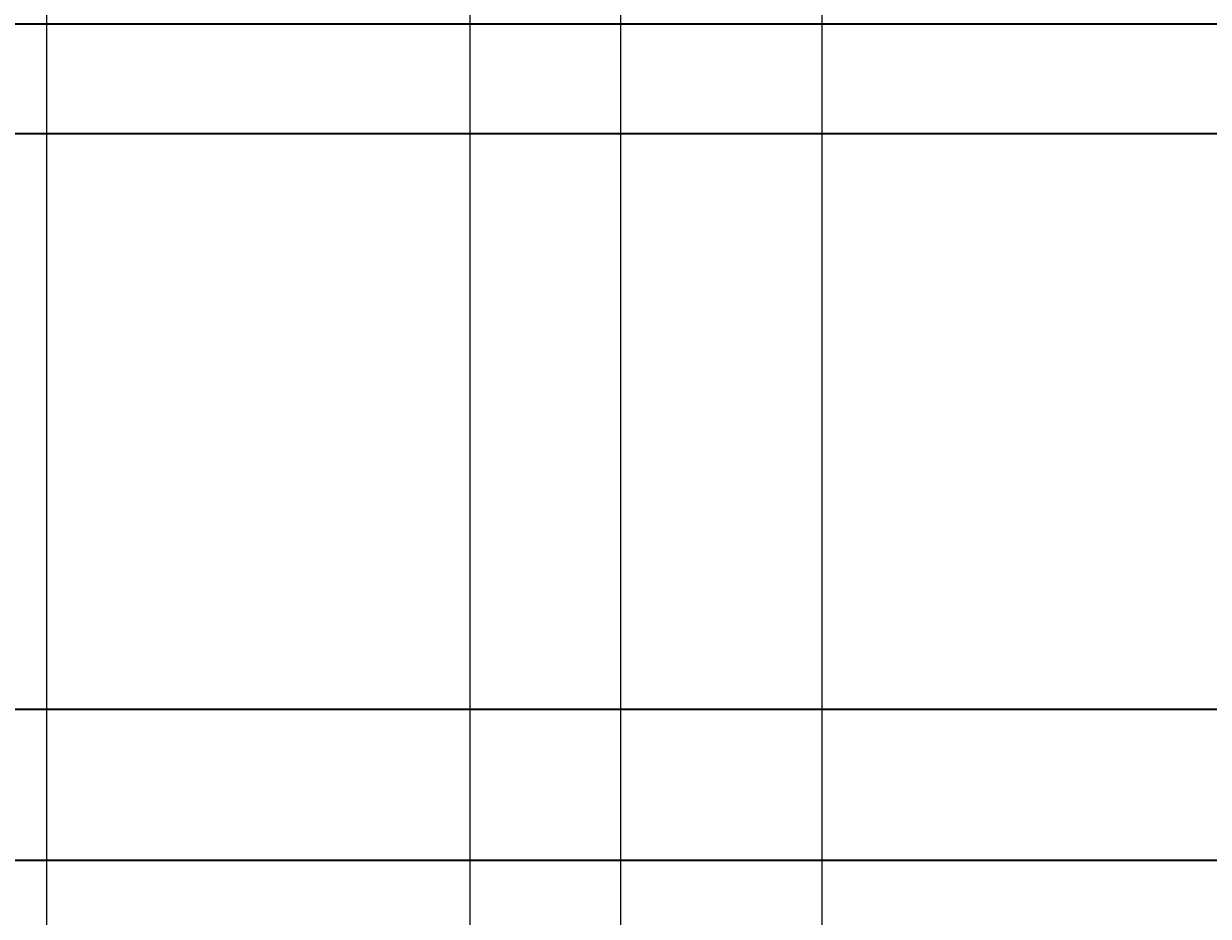
# Model space of a CAD drawing. Units: inches. Extents: x -6 to 289, y -8 to 323.
# Tile 86 of 107: x 126 to 150, y 276 to 294. Entities that reach past the tile are written whole.
import ezdxf

# ---------------------------------------------------------------- set-up
doc = ezdxf.new("R2010")
doc.units = ezdxf.units.IN
doc.header["$MEASUREMENT"] = 0
doc.layers.add('A-ANNO-DIMS', color=2, linetype='Continuous', lineweight=18)
doc.layers.add('A-ELEV', color=7, linetype='Continuous', lineweight=35)
doc.styles.get("Standard").update_dxf_attribs({"font": 'arial.ttf'})
doc.dimstyles.get("Standard").update_dxf_attribs({"dimtxt": 0.18, "dimasz": 0.18, "dimexe": 0.18, "dimexo": 0.0625, "dimgap": 0.09, "dimtad": 0, "dimtih": 1, "dimtoh": 1, "dimdec": 4, "dimzin": 0, "dimdsep": 46, "dimtxsty": 'Standard', "dimcen": 0.09, "dimadec": 0, "dimazin": 0, "dimtfac": 1, "dimtdec": 4, "dimtofl": 0, "dimtmove": 0, "dimatfit": 3, "dimfxl": 1, "dimtolj": 1, "dimtzin": 0, "dimarcsym": 0})

# ---------------------------------------------------------------- blocks, each defined once
blk = doc.blocks.new('*D10')
at = {"layer": 'A-ANNO-DIMS', "color": 0, "lineweight": -2, "transparency": 16777216}
for p, q in [((115.164, 307.351), (115.164, 322.969)), ((126.883, 226.717), (126.883, 322.969)), ((115.344, 322.789), (120.639, 322.789)), ((126.703, 322.789), (121.408, 322.789))]:
    blk.add_line(p, q, dxfattribs=at)
at = {"layer": 'A-ANNO-DIMS', "color": 0, "transparency": 16777216}
for points in [[(115.344, 322.819), (115.344, 322.759), (115.164, 322.789)], [(126.703, 322.819), (126.703, 322.759), (126.883, 322.789)]]:
    blk.add_solid(points, dxfattribs=at)
at = {"layer": 'Defpoints', "color": 0, "transparency": 16777216}
for p in [(126.883, 322.789), (115.164, 307.289), (126.883, 226.654)]:
    blk.add_point(p, dxfattribs=at)
at = {"layer": 'A-ANNO-DIMS', "color": 0, "transparency": 16777216, "insert": (121.024, 322.789), "char_height": 0.18, "attachment_point": 5}
blk.add_mtext('\\A1;11.72', dxfattribs=at)
blk = doc.blocks.new('*D11')
at = {"layer": 'A-ANNO-DIMS', "color": 0, "lineweight": -2, "transparency": 16777216}
for p, q in [((126.883, 226.717), (126.883, 322.969)), ((168.883, 226.717), (168.883, 322.969)), ((127.063, 322.789), (147.662, 322.789)), ((168.703, 322.789), (148.105, 322.789))]:
    blk.add_line(p, q, dxfattribs=at)
at = {"layer": 'A-ANNO-DIMS', "color": 0, "transparency": 16777216}
for points in [[(127.063, 322.819), (127.063, 322.759), (126.883, 322.789)], [(168.703, 322.819), (168.703, 322.759), (168.883, 322.789)]]:
    blk.add_solid(points, dxfattribs=at)
at = {"layer": 'Defpoints', "color": 0, "transparency": 16777216}
for p in [(168.883, 322.789), (126.883, 226.654), (168.883, 226.654)]:
    blk.add_point(p, dxfattribs=at)
at = {"layer": 'A-ANNO-DIMS', "color": 0, "transparency": 16777216, "insert": (147.883, 322.789), "char_height": 0.18, "attachment_point": 5}
blk.add_mtext('\\A1;42', dxfattribs=at)
blk = doc.blocks.new('*D27')
at = {"layer": 'A-ANNO-DIMS', "color": 0, "lineweight": -2, "transparency": 16777216}
for p, q in [((19.226, 307.289), (288.653, 307.289)), ((288.473, 307.109), (288.473, 277.471)), ((288.473, 247.469), (288.473, 277.107)), ((247.226, 247.289), (288.653, 247.289))]:
    blk.add_line(p, q, dxfattribs=at)
at = {"layer": 'A-ANNO-DIMS', "color": 0, "transparency": 16777216}
for points in [[(288.443, 307.109), (288.503, 307.109), (288.473, 307.289)], [(288.443, 247.469), (288.503, 247.469), (288.473, 247.289)]]:
    blk.add_solid(points, dxfattribs=at)
at = {"layer": 'Defpoints', "color": 0, "transparency": 16777216}
for p in [(19.164, 307.289), (288.473, 307.289), (247.164, 247.289)]:
    blk.add_point(p, dxfattribs=at)
at = {"layer": 'A-ANNO-DIMS', "color": 0, "transparency": 16777216, "insert": (288.473, 277.289), "char_height": 0.18, "attachment_point": 5}
blk.add_mtext('\\A1;60', dxfattribs=at)
blk = doc.blocks.new('*D73')
at = {"layer": 'A-ANNO-DIMS', "color": 0, "lineweight": -2, "transparency": 16777216}
for p, q in [((121.008, 51.148), (121.008, 322.969)), ((135.296, 51.148), (135.296, 322.969)), ((121.188, 322.789), (127.697, 322.789)), ((135.116, 322.789), (128.607, 322.789))]:
    blk.add_line(p, q, dxfattribs=at)
at = {"layer": 'A-ANNO-DIMS', "color": 0, "transparency": 16777216}
for points in [[(121.188, 322.819), (121.188, 322.759), (121.008, 322.789)], [(135.116, 322.819), (135.116, 322.759), (135.296, 322.789)]]:
    blk.add_solid(points, dxfattribs=at)
at = {"layer": 'Defpoints', "color": 0, "transparency": 16777216}
for p in [(135.296, 322.789), (121.008, 51.085), (135.296, 51.085)]:
    blk.add_point(p, dxfattribs=at)
at = {"layer": 'A-ANNO-DIMS', "color": 0, "transparency": 16777216, "insert": (128.152, 322.789), "char_height": 0.18, "attachment_point": 5}
blk.add_mtext('\\A1;14.288', dxfattribs=at)
blk = doc.blocks.new('*D74')
at = {"layer": 'A-ANNO-DIMS', "color": 0, "lineweight": -2, "transparency": 16777216}
for p, q in [((135.296, 51.148), (135.296, 322.969)), ((138.296, 51.148), (138.296, 322.969)), ((135.476, 322.789), (136.647, 322.789)), ((138.116, 322.789), (136.945, 322.789))]:
    blk.add_line(p, q, dxfattribs=at)
at = {"layer": 'A-ANNO-DIMS', "color": 0, "transparency": 16777216}
for points in [[(135.476, 322.819), (135.476, 322.759), (135.296, 322.789)], [(138.116, 322.819), (138.116, 322.759), (138.296, 322.789)]]:
    blk.add_solid(points, dxfattribs=at)
at = {"layer": 'Defpoints', "color": 0, "transparency": 16777216}
for p in [(138.296, 322.789), (135.296, 51.085), (138.296, 51.085)]:
    blk.add_point(p, dxfattribs=at)
at = {"layer": 'A-ANNO-DIMS', "color": 0, "transparency": 16777216, "insert": (136.796, 322.789), "char_height": 0.18, "attachment_point": 5}
blk.add_mtext('\\A1;3', dxfattribs=at)
blk = doc.blocks.new('*D75')
at = {"layer": 'A-ANNO-DIMS', "color": 0, "lineweight": -2, "transparency": 16777216}
for p, q in [((138.296, 51.148), (138.296, 322.969)), ((142.296, 51.148), (142.296, 322.969)), ((138.476, 322.789), (140.144, 322.789)), ((142.116, 322.789), (140.448, 322.789))]:
    blk.add_line(p, q, dxfattribs=at)
at = {"layer": 'A-ANNO-DIMS', "color": 0, "transparency": 16777216}
for points in [[(138.476, 322.819), (138.476, 322.759), (138.296, 322.789)], [(142.116, 322.819), (142.116, 322.759), (142.296, 322.789)]]:
    blk.add_solid(points, dxfattribs=at)
at = {"layer": 'Defpoints', "color": 0, "transparency": 16777216}
for p in [(142.296, 322.789), (138.296, 51.085), (142.296, 51.085)]:
    blk.add_point(p, dxfattribs=at)
at = {"layer": 'A-ANNO-DIMS', "color": 0, "transparency": 16777216, "insert": (140.296, 322.789), "char_height": 0.18, "attachment_point": 5}
blk.add_mtext('\\A1;4', dxfattribs=at)
blk = doc.blocks.new('*D76')
at = {"layer": 'A-ANNO-DIMS', "color": 0, "lineweight": -2, "transparency": 16777216}
for p, q in [((142.296, 51.148), (142.296, 322.969)), ((164.296, 51.148), (164.296, 322.969)), ((142.476, 322.789), (153.076, 322.789)), ((164.116, 322.789), (153.516, 322.789))]:
    blk.add_line(p, q, dxfattribs=at)
at = {"layer": 'A-ANNO-DIMS', "color": 0, "transparency": 16777216}
for points in [[(142.476, 322.819), (142.476, 322.759), (142.296, 322.789)], [(164.116, 322.819), (164.116, 322.759), (164.296, 322.789)]]:
    blk.add_solid(points, dxfattribs=at)
at = {"layer": 'Defpoints', "color": 0, "transparency": 16777216}
for p in [(164.296, 322.789), (142.296, 51.085), (164.296, 51.085)]:
    blk.add_point(p, dxfattribs=at)
at = {"layer": 'A-ANNO-DIMS', "color": 0, "transparency": 16777216, "insert": (153.296, 322.789), "char_height": 0.18, "attachment_point": 5}
blk.add_mtext('\\A1;22', dxfattribs=at)
blk = doc.blocks.new('*D94')
at = {"layer": 'A-ANNO-DIMS', "color": 0, "lineweight": -2, "transparency": 16777216}
for p, q in [((118.164, 159.411), (118.164, 322.969)), ((161.552, 159.411), (161.552, 322.969)), ((118.344, 322.789), (139.46, 322.789)), ((161.372, 322.789), (140.256, 322.789))]:
    blk.add_line(p, q, dxfattribs=at)
at = {"layer": 'A-ANNO-DIMS', "color": 0, "transparency": 16777216}
for points in [[(118.344, 322.819), (118.344, 322.759), (118.164, 322.789)], [(161.372, 322.819), (161.372, 322.759), (161.552, 322.789)]]:
    blk.add_solid(points, dxfattribs=at)
at = {"layer": 'Defpoints', "color": 0, "transparency": 16777216}
for p in [(161.552, 322.789), (118.164, 159.348), (161.552, 159.348)]:
    blk.add_point(p, dxfattribs=at)
at = {"layer": 'A-ANNO-DIMS', "color": 0, "transparency": 16777216, "insert": (139.858, 322.789), "char_height": 0.18, "attachment_point": 5}
blk.add_mtext('\\A1;43.39', dxfattribs=at)
blk = doc.blocks.new('*D107')
at = {"layer": 'A-ANNO-DIMS', "color": 0, "lineweight": -2, "transparency": 16777216}
for p, q in [((118.164, 293.728), (118.164, 322.969)), ((186.984, 291.541), (186.984, 322.969)), ((118.344, 322.789), (152.18, 322.789)), ((186.804, 322.789), (152.967, 322.789))]:
    blk.add_line(p, q, dxfattribs=at)
at = {"layer": 'A-ANNO-DIMS', "color": 0, "transparency": 16777216}
for points in [[(118.344, 322.819), (118.344, 322.759), (118.164, 322.789)], [(186.804, 322.819), (186.804, 322.759), (186.984, 322.789)]]:
    blk.add_solid(points, dxfattribs=at)
at = {"layer": 'Defpoints', "color": 0, "transparency": 16777216}
for p in [(186.984, 322.789), (118.164, 293.666), (186.984, 291.478)]:
    blk.add_point(p, dxfattribs=at)
at = {"layer": 'A-ANNO-DIMS', "color": 0, "transparency": 16777216, "insert": (152.574, 322.789), "char_height": 0.18, "attachment_point": 5}
blk.add_mtext('\\A1;68.82', dxfattribs=at)

msp = doc.modelspace()

# ---------------------------------------------------------------- linework, layer by layer
at = {"layer": 'A-ELEV'}
for points in [[(115.1638, 307.2888), (115.1638, 277.0427), (259.1638, 277.0427), (259.1638, 259.2888)], [(118.1638, 307.2888), (118.1638, 280.0427), (262.1638, 280.0427), (262.1638, 259.2888)], [(255.8036, 291.4781), (118.1638, 291.4781), (118.1638, 293.6657), (255.8036, 293.6657)]]:
    msp.add_lwpolyline(points, dxfattribs=at)

# ---------------------------------------------------------------- dimensions: what is measured, and where the dimension line sits
at = {"layer": 'A-ANNO-DIMS'}
for base, p1, p2, override, picture, middle in [((126.8835, 322.7888), (115.1638, 307.2888), (126.8835, 226.654), {"dimdec": 2, "dimlfac": 1, "dimrnd": 0, "dimzin": 0, "dimdsep": 46, "dimlunit": 2}, '*D10', (121.0236, 322.7888)), ((161.5522, 322.7888), (118.1638, 159.3484), (161.5522, 159.3484), {"dimdec": 2, "dimlfac": 1, "dimrnd": 0, "dimzin": 0, "dimdsep": 46, "dimlunit": 2}, '*D94', (139.858, 322.7888)), ((186.9837, 322.7888), (118.1638, 293.6657), (186.9837, 291.4781), {"dimdec": 2, "dimlfac": 1, "dimrnd": 0, "dimzin": 0, "dimdsep": 46, "dimlunit": 2}, '*D107', (152.5737, 322.7888)), ((135.296, 322.7888), (121.008, 51.0851), (135.296, 51.0851), {"dimdec": 3, "dimlfac": 1, "dimrnd": 0, "dimzin": 0, "dimdsep": 46, "dimlunit": 2}, '*D73', (128.152, 322.7888)), ((168.8835, 322.7888), (126.8835, 226.654), (168.8835, 226.654), {"dimdec": 0, "dimlfac": 1, "dimrnd": 0, "dimzin": 0, "dimdsep": 46, "dimlunit": 2}, '*D11', (147.8835, 322.7888)), ((138.296, 322.7888), (135.296, 51.0851), (138.296, 51.0851), {"dimdec": 0, "dimlfac": 1, "dimrnd": 0, "dimzin": 0, "dimdsep": 46, "dimlunit": 2}, '*D74', (136.796, 322.7888)), ((142.296, 322.7888), (138.296, 51.0851), (142.296, 51.0851), {"dimdec": 0, "dimlfac": 1, "dimrnd": 0, "dimzin": 0, "dimdsep": 46, "dimlunit": 2}, '*D75', (140.296, 322.7888)), ((164.296, 322.7888), (142.296, 51.0851), (164.296, 51.0851), {"dimdec": 0, "dimlfac": 1, "dimrnd": 0, "dimzin": 0, "dimdsep": 46, "dimlunit": 2}, '*D76', (153.296, 322.7888))]:
    dim = msp.add_linear_dim(base=base, p1=p1, p2=p2, dimstyle='Standard', override=override, dxfattribs=at)
    dim.commit()
    dim.dimension.update_dxf_attribs({"geometry": picture, "text_midpoint": middle})
dim = msp.add_linear_dim(base=(288.4733, 307.2888), p1=(247.1638, 247.2888), p2=(19.1638, 307.2888), angle=90, dimstyle='Standard', override={"dimdec": 0, "dimlfac": 1, "dimrnd": 0, "dimzin": 0, "dimdsep": 46, "dimlunit": 2}, dxfattribs=at)
dim.commit()
dim.dimension.update_dxf_attribs({"geometry": '*D27', "text_midpoint": (288.4733, 277.2888)})

doc.saveas('drawing.dxf')
